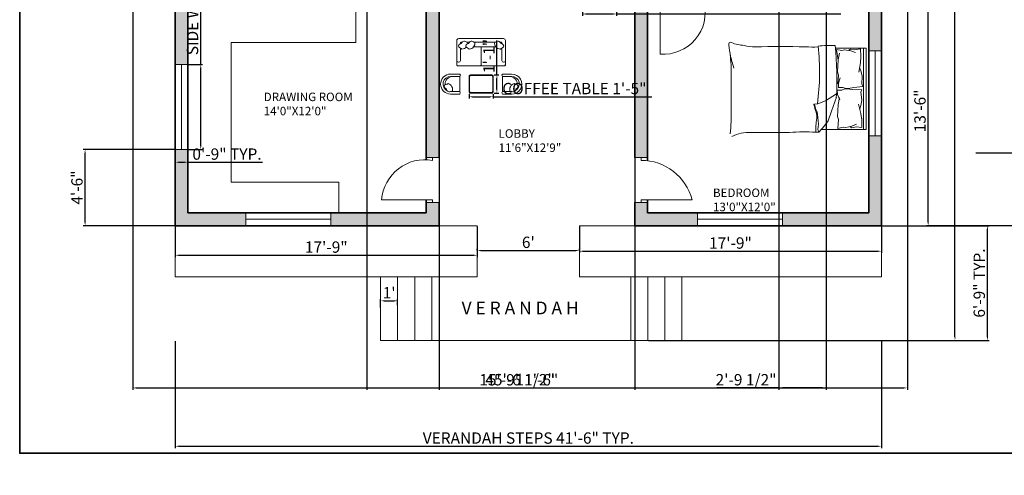
# Model space of a CAD drawing. Units: inches. Extents: x 2257 to 3678, y 834 to 1975.
# Tile 1 of 16: x 2257 to 2952, y 834 to 1155. Entities that reach past the tile are written whole.
import ezdxf

# ---------------------------------------------------------------- set-up
doc = ezdxf.new("R2010")
doc.units = ezdxf.units.IN
for name, color, linetype, lineweight in [('A-ANNO-DIMS', 2, 'Continuous', 18), ('A-ANNO-SYMB', 7, 'Continuous', 25), ('A-ANNO-TTLB', 7, 'Continuous', 35), ('A-AREA-IDEN', 7, 'Continuous', 18), ('A-DOOR', 3, 'Continuous', 18), ('A-FLOR-CASE', 8, 'Continuous', 18), ('A-FLOR-STRS', 7, 'Continuous', 18), ('A-FURN', 8, 'Continuous', 18), ('A-GLAZ', 4, 'Continuous', 18), ('A-WALL', 7, 'Continuous', 35)]:
    doc.layers.add(name, color=color, linetype=linetype, lineweight=lineweight)
doc.layers.add('A-WALL-PATT', color=251, linetype='Continuous', lineweight=13, true_color=0x636466)
doc.styles.get("Standard").update_dxf_attribs({"font": 'arial.ttf'})
doc.dimstyles.new('ISO-25', dxfattribs={"dimtxt": 8, "dimasz": 2.5, "dimexe": 1.25, "dimexo": 0.625, "dimtad": 1, "dimdec": 0, "dimlunit": 3, "dimtxsty": 'Standard', "dimcen": 2.5, "dimadec": 0, "dimazin": 0, "dimtfac": 1, "dimtdec": 0, "dimtmove": 0, "dimatfit": 3, "dimfxl": 1, "dimarcsym": 0})

# ---------------------------------------------------------------- blocks, each defined once
blk = doc.blocks.new('*D7')
at = {"layer": 'A-ANNO-DIMS', "color": 0, "lineweight": -2, "transparency": 16777216}
for p, q in [((2367.05, 1009.45), (2367.05, 987.96)), ((2580.05, 1009.45), (2580.05, 987.96)), ((2369.55, 989.21), (2577.55, 989.21))]:
    blk.add_line(p, q, dxfattribs=at)
at = {"layer": 'A-ANNO-DIMS', "color": 0, "transparency": 16777216}
for points in [[(2369.55, 989.62), (2369.55, 988.79), (2367.05, 989.21)], [(2577.55, 989.62), (2577.55, 988.79), (2580.05, 989.21)]]:
    blk.add_solid(points, dxfattribs=at)
at = {"layer": 'Defpoints', "color": 0, "transparency": 16777216}
for p in [(2367.05, 1010.08), (2580.05, 1010.08), (2580.05, 989.21)]:
    blk.add_point(p, dxfattribs=at)
at = {"layer": 'A-ANNO-DIMS', "color": 0, "transparency": 16777216, "insert": (2473.55, 993.92), "char_height": 8, "attachment_point": 5}
blk.add_mtext('17\'-9"', dxfattribs=at)
blk = doc.blocks.new('*D8')
at = {"layer": 'A-ANNO-DIMS', "color": 0, "lineweight": -2, "transparency": 16777216}
for p, q in [((2652.05, 1009.45), (2652.05, 990.83)), ((2865.05, 1009.45), (2865.05, 990.83)), ((2654.55, 992.08), (2862.55, 992.08))]:
    blk.add_line(p, q, dxfattribs=at)
at = {"layer": 'A-ANNO-DIMS', "color": 0, "transparency": 16777216}
for points in [[(2654.55, 992.49), (2654.55, 991.66), (2652.05, 992.08)], [(2862.55, 992.49), (2862.55, 991.66), (2865.05, 992.08)]]:
    blk.add_solid(points, dxfattribs=at)
at = {"layer": 'Defpoints', "color": 0, "transparency": 16777216}
for p in [(2652.05, 1010.08), (2865.05, 1010.08), (2865.05, 992.08)]:
    blk.add_point(p, dxfattribs=at)
at = {"layer": 'A-ANNO-DIMS', "color": 0, "transparency": 16777216, "insert": (2758.55, 996.79), "char_height": 8, "attachment_point": 5}
blk.add_mtext('17\'-9"', dxfattribs=at)
blk = doc.blocks.new('*D9')
at = {"layer": 'A-ANNO-DIMS', "color": 0, "lineweight": -2, "transparency": 16777216}
for p, q in [((2580.05, 992.7), (2580.05, 993.82)), ((2652.05, 992.7), (2652.05, 993.82)), ((2582.55, 992.57), (2649.55, 992.57))]:
    blk.add_line(p, q, dxfattribs=at)
at = {"layer": 'A-ANNO-DIMS', "color": 0, "transparency": 16777216}
for points in [[(2582.55, 992.99), (2582.55, 992.16), (2580.05, 992.57)], [(2649.55, 992.99), (2649.55, 992.16), (2652.05, 992.57)]]:
    blk.add_solid(points, dxfattribs=at)
at = {"layer": 'Defpoints', "color": 0, "transparency": 16777216}
for p in [(2580.05, 992.08), (2652.05, 992.57), (2652.05, 992.08)]:
    blk.add_point(p, dxfattribs=at)
at = {"layer": 'A-ANNO-DIMS', "color": 0, "transparency": 16777216, "insert": (2616.05, 997.28), "char_height": 8, "attachment_point": 5}
blk.add_mtext("6'", dxfattribs=at)
blk = doc.blocks.new('A$C1352')
at = {"color": 0}
for points in [[(0.003, 0.053), (0.003, 0.553, -0.414214), (0.053, 0.603), (0.753, 0.603, -0.414214), (0.803, 0.553), (0.803, 0.053, -0.414214), (0.753, 0.003), (0.053, 0.003, -0.414214)], [(0.023, 0.053), (0.023, 0.553, -0.414214), (0.053, 0.583), (0.753, 0.583, -0.414214), (0.783, 0.553), (0.783, 0.053, -0.414214), (0.753, 0.023), (0.053, 0.023, -0.414214)]]:
    blk.add_lwpolyline(points, format="xyb", close=True, dxfattribs=at)
blk = doc.blocks.new('*D21')
at = {"layer": 'A-ANNO-DIMS', "color": 0, "lineweight": -2, "transparency": 16777216}
for p, q in [((2511.89, 952.22), (2511.89, 958.28)), ((2523.89, 953.88), (2523.89, 958.28)), ((2514.39, 957.03), (2521.39, 957.03))]:
    blk.add_line(p, q, dxfattribs=at)
at = {"layer": 'A-ANNO-DIMS', "color": 0, "transparency": 16777216}
for points in [[(2514.39, 957.45), (2514.39, 956.61), (2511.89, 957.03)], [(2521.39, 957.45), (2521.39, 956.61), (2523.89, 957.03)]]:
    blk.add_solid(points, dxfattribs=at)
at = {"layer": 'Defpoints', "color": 0, "transparency": 16777216}
for p in [(2511.89, 951.59), (2523.89, 957.03), (2523.89, 953.26)]:
    blk.add_point(p, dxfattribs=at)
at = {"layer": 'A-ANNO-DIMS', "color": 0, "transparency": 16777216, "insert": (2517.89, 961.67), "char_height": 8, "attachment_point": 5}
blk.add_mtext("1'", dxfattribs=at)
blk = doc.blocks.new('BED-DOUBLE-PLAN')
for p, q in [((33.26, 63.38), (29.37, 58.94)), ((35.36, 63.48), (33.26, 63.38, 4.64)), ((34.01, 61.54), (33.26, 63.38)), ((0, 61.46), (31.9, 61.46)), ((0, 4.17), (0, 61.46)), ((1.84, 4.17), (1.84, 61.46)), ((3.07, 60.08), (2.95, 53.6)), ((3.07, 60.08), (6.92, 59.62)), ((9.9, 59.11), (6.69, 57.7)), ((6.92, 59.62), (10, 60.34)), ((14.18, 60.08), (9.9, 59.11)), ((10, 60.34), (11.25, 59.72)), ((16.11, 59.85), (14.18, 60.08)), ((19.87, 60.78), (16.11, 59.85)), ((19.38, 54.63), (19.87, 60.78)), ((29.37, 58.94), (26.77, 55.41)), ((33.63, 57.82), (34.01, 61.54)), ((34.01, 53.18), (33.63, 57.82)), ((2.95, 53.6), (3.05, 54.8)), ((3.05, 54.8), (3.68, 50.25)), ((3.68, 50.25), (5.3, 43.75)), ((20.05, 52.28), (19.38, 54.63)), ((19.54, 43.87), (20.05, 52.28)), ((24.36, 48.73), (20.84, 38.73)), ((26.77, 55.41), (24.36, 48.73)), ((34.56, 49.1), (34.01, 53.18)), ((35.68, 46.68), (34.56, 49.1)), ((3.69, 44.52), (3.04, 41.01)), ((4.4, 47), (3.69, 44.52)), ((18.74, 39.04), (19.54, 43.87)), ((28.62, 41.3), (34.01, 43.34)), ((34.01, 43.34), (36.42, 43.71)), ((36.42, 43.71), (35.68, 46.68)), ((95, 18.06), (95, 47.57)), ((3.57, 35.31), (2.99, 33.54)), ((3.04, 41.01), (3.07, 40.62)), ((3.07, 40.62), (3.57, 35.31)), ((20.07, 36.86), (18.53, 40.55)), ((20.25, 33.92), (20.07, 36.86)), ((20.84, 36.28), (28.62, 41.3)), ((2.24, 31.15), (8.66, 31.84)), ((2.94, 29.42), (2.24, 31.15)), ((2.76, 24.09), (2.94, 29.42)), ((2.99, 33.54), (9.43, 33.25)), ((8.66, 31.84), (12.47, 32.54)), ((9.43, 33.25), (13.28, 32.79)), ((12.47, 32.54), (14.03, 32.54)), ((13.28, 32.79), (14.84, 32.89)), ((14.03, 32.54), (16.28, 31.84)), ((14.84, 32.89), (17.04, 33.72)), ((16.28, 31.84), (19.5, 31.84)), ((17.04, 33.72), (20.25, 33.92)), ((19.5, 28.9), (18.19, 25.13)), ((19.38, 23.24), (19.87, 29.39)), ((19.5, 31.84), (19.5, 28.9)), ((2.76, 23.7), (2.76, 24.09)), ((3.63, 20.23), (2.76, 23.7)), ((3.98, 14.52), (5.19, 21.1)), ((20.05, 20.89), (19.38, 23.24)), ((19.54, 12.48), (20.05, 20.89)), ((4.5, 17.81), (3.63, 20.23)), ((3.63, 9.93), (3.98, 14.52)), ((3.61, 9.81), (3.63, 9.93)), ((4, 4.67), (3.61, 9.81)), ((10.74, 6.06), (7.44, 7.27)), ((18.74, 7.65), (19.54, 12.48)), ((19.54, 12.48), (19.92, 11.13)), ((19.92, 11.13), (20.79, 5.02)), ((21.71, 4.17), (0, 4.17)), ((3.98, 4.67), (7.79, 5.36)), ((7.79, 5.36), (10.91, 4.84)), ((15.07, 5.36), (10.74, 6.06)), ((10.91, 4.84), (12.12, 5.54)), ((16.98, 5.71), (15.07, 5.36)), ((20.79, 5.02), (16.98, 5.71))]:
    blk.add_line(p, q)
for centre, radius, start, end in [((-7.98, 61.53), 43.38, 349.87628, 2.56571), ((43.54, 218.51), 155.25, 266.97912, 273.83645), ((81.31, -5405.34), 5469.02, 90.00217, 90.28689), ((82.32, 91.3), 27.65, 267.47136, 296.46809), ((254.49, 49.33), 159.5, 174.4998, 180.63509), ((42.04, 52.44), 7.46, 168.6608, 203.73842), ((1.78, 37.35), 35.55, 10.66171, 19.88058), ((187.4, 21.29), 154.68, 171.78449, 186.90062), ((36.49, 43.92), 0.221, 250.24637, 1.13765), ((218.26, 25.61), 197.77, 176.08655, 186.78213), ((-28.43, -20.65), 127.63, 13.38322, 17.70533), ((240.78, 25.69), 145.97, 182.99578, 189.40907), ((24.09, 102.1), 99.87, 268.72178, 275.60397), ((37.37, -200.58), 203.94, 88.4762, 91.00819), ((60.68, 581.23), 578.22, 268.22771, 271.71854), ((77.34, -32.25), 35.53, 76.06484, 88.91125), ((84.25, -25.97), 28.25, 67.97508, 86.652), ((95.57, 1.3), 1.31, 236.17358, 23.47814)]:
    blk.add_arc(centre, radius, start, end)
blk = doc.blocks.new('WIN-60')
for p, q in [((0, 9), (0, 0)), ((60, 4.5), (60, 9)), ((60, 9), (60, 0)), ((0, 0), (0, 4.5)), ((0, 4.5), (60, 4.5))]:
    blk.add_line(p, q)
blk = doc.blocks.new('WIN-60-SIDE')
for p, q in [((0, 60), (9, 60)), ((9, 60), (4.5, 60)), ((4.5, 60), (4.5, 0)), ((9, 0), (0, 0)), ((4.5, 0), (9, 0))]:
    blk.add_line(p, q)
blk = doc.blocks.new('DOOR-BEDROOM-FRONT')
for p, q in [((0, 41.01), (0, 32.01)), ((0, 36.08), (2, 36.08)), ((2, 36.08), (2, 0.08)), ((34.84, 36.51), (32.84, 36.51)), ((34.84, 41.01), (34.84, 32.01)), ((34.84, 32.01), (34.84, 36.51))]:
    blk.add_line(p, q)
blk.add_arc((4.15, 29.52), 29.53, 265.82197, 13.68707)
blk = doc.blocks.new('DOOR-DRAWING-ROOM')
for p, q in [((31.5, 31.83), (40.5, 31.83)), ((40.5, 31.83), (36, 31.83)), ((36, 31.83), (36, 29.83)), ((36, 2), (0, 2)), ((36, 0), (36, 2)), ((31.5, 0), (40.5, 0)), ((40.5, 0), (36, 0))]:
    blk.add_line(p, q)
blk.add_arc((30.7, -0.52), 30.81, 80.10035, 175.31629)
blk = doc.blocks.new('DOOR-LOBBY-BEDROOM')
for p, q in [((0, 31.83), (9, 31.83)), ((9, 31.83), (4.5, 31.83)), ((4.5, 31.83), (4.5, 29.83)), ((4.5, 0), (4.5, 2)), ((4.5, 2), (40.5, 2)), ((0, 0), (0, 0)), ((0, 0), (9, 0)), ((9, 0), (4.5, 0))]:
    blk.add_line(p, q)
blk.add_arc((4.5, -7.37), 37.2, 14.58337, 90)
blk = doc.blocks.new('STEPS-VERANDAH')
for p, q in [((0, 80.97), (213, 80.97)), ((0, 44.97), (0, 80.97)), ((0, 80.97), (0, 80.97)), ((213, 80.97), (213, 44.97)), ((213, 80.97), (213, 44.97)), ((498, 80.97), (285, 80.97)), ((285, 80.97), (285, 44.97)), ((285, 80.97), (285, 44.97)), ((498, 44.97), (498, 80.97)), ((213, 44.97), (0, 44.97)), ((144.84, 0), (144.84, 44.97)), ((168.84, 44.97), (156.84, 44.97)), ((156.84, 44.97), (156.84, 0)), ((168.84, 0), (168.84, 44.97)), ((168.84, 44.97), (168.84, 44.97)), ((180.84, 44.97), (180.84, 0)), ((285, 44.97), (498, 44.97)), ((333.2, 44.97), (321.2, 44.97)), ((321.2, 44.97), (321.2, 0)), ((333.2, 0), (333.2, 44.97)), ((357.2, 44.97), (345.2, 44.97)), ((345.2, 44.97), (345.2, 0)), ((357.2, 0), (357.2, 44.97)), ((213, 0), (144.84, 0)), ((156.84, 0), (144.84, 0)), ((180.84, 0), (168.84, 0)), ((213, 0), (357.2, 0)), ((345.2, 0), (333.2, 0))]:
    blk.add_line(p, q)
blk = doc.blocks.new('*D54')
at = {"layer": 'A-ANNO-DIMS', "color": 0, "lineweight": -2, "transparency": 16777216}
for p, q in [((2574.2, 1102.98), (2574.2, 1099.79)), ((2576.7, 1101.04), (2588.83, 1101.04)), ((2591.33, 1102.98), (2591.33, 1099.79)), ((2591.33, 1101.04), (2703.2, 1101.04))]:
    blk.add_line(p, q, dxfattribs=at)
at = {"layer": 'A-ANNO-DIMS', "color": 0, "transparency": 16777216}
for points in [[(2576.7, 1101.45), (2576.7, 1100.62), (2574.2, 1101.04)], [(2588.83, 1101.45), (2588.83, 1100.62), (2591.33, 1101.04)]]:
    blk.add_solid(points, dxfattribs=at)
at = {"layer": 'Defpoints', "color": 0, "transparency": 16777216}
for p in [(2574.2, 1103.61), (2591.33, 1103.61), (2591.33, 1101.04)]:
    blk.add_point(p, dxfattribs=at)
at = {"layer": 'A-ANNO-DIMS', "color": 0, "transparency": 16777216, "insert": (2648.51, 1105.8), "char_height": 8, "attachment_point": 5}
blk.add_mtext('COFFEE TABLE 1\'-5"', dxfattribs=at)
blk = doc.blocks.new('*D55')
at = {"layer": 'A-ANNO-DIMS', "color": 0, "lineweight": -2, "transparency": 16777216}
for p, q in [((2593.9, 1116.46), (2593.9, 1140.72)), ((2591.96, 1116.46), (2595.15, 1116.46)), ((2593.9, 1106.11), (2593.9, 1113.96)), ((2591.96, 1103.61), (2595.15, 1103.61))]:
    blk.add_line(p, q, dxfattribs=at)
at = {"layer": 'A-ANNO-DIMS', "color": 0, "transparency": 16777216}
for points in [[(2593.49, 1113.96), (2594.32, 1113.96), (2593.9, 1116.46)], [(2593.49, 1106.11), (2594.32, 1106.11), (2593.9, 1103.61)]]:
    blk.add_solid(points, dxfattribs=at)
at = {"layer": 'Defpoints', "color": 0, "transparency": 16777216}
for p in [(2591.33, 1116.46), (2593.9, 1116.46), (2591.33, 1103.61)]:
    blk.add_point(p, dxfattribs=at)
at = {"layer": 'A-ANNO-DIMS', "color": 0, "transparency": 16777216, "insert": (2589.26, 1129.84), "char_height": 8, "attachment_point": 5, "rotation": 90}
blk.add_mtext('1\'-1"', dxfattribs=at)
blk = doc.blocks.new('*D58')
at = {"layer": 'A-ANNO-DIMS', "color": 0, "lineweight": -2, "transparency": 16777216}
for p, q in [((2385.05, 1123.86), (2385.05, 1257.67)), ((2376.68, 1123.86), (2386.3, 1123.86)), ((2385.05, 1066.36), (2385.05, 1121.36)), ((2376.68, 1063.86), (2386.3, 1063.86))]:
    blk.add_line(p, q, dxfattribs=at)
at = {"layer": 'A-ANNO-DIMS', "color": 0, "transparency": 16777216}
for points in [[(2384.63, 1121.36), (2385.47, 1121.36), (2385.05, 1123.86)], [(2384.63, 1066.36), (2385.47, 1066.36), (2385.05, 1063.86)]]:
    blk.add_solid(points, dxfattribs=at)
at = {"layer": 'Defpoints', "color": 0, "transparency": 16777216}
for p in [(2376.05, 1123.86), (2385.05, 1123.86), (2376.05, 1063.86)]:
    blk.add_point(p, dxfattribs=at)
at = {"layer": 'A-ANNO-DIMS', "color": 0, "transparency": 16777216, "insert": (2380.29, 1192.01), "char_height": 8, "attachment_point": 5, "rotation": 90}
blk.add_mtext('SIDE WINDOW 5\'-0" TYP.', dxfattribs=at)
blk = doc.blocks.new('*D59')
at = {"layer": 'A-ANNO-DIMS', "color": 0, "lineweight": -2, "transparency": 16777216}
for p, q in [((2367.05, 1063.23), (2367.05, 1053.61)), ((2376.05, 1063.23), (2376.05, 1053.61)), ((2369.55, 1054.86), (2373.55, 1054.86)), ((2376.05, 1054.86), (2428.56, 1054.86))]:
    blk.add_line(p, q, dxfattribs=at)
at = {"layer": 'A-ANNO-DIMS', "color": 0, "transparency": 16777216}
for points in [[(2369.55, 1055.28), (2369.55, 1054.44), (2367.05, 1054.86)], [(2373.55, 1055.28), (2373.55, 1054.44), (2376.05, 1054.86)]]:
    blk.add_solid(points, dxfattribs=at)
at = {"layer": 'Defpoints', "color": 0, "transparency": 16777216}
for p in [(2367.05, 1063.86), (2376.05, 1063.86), (2376.05, 1054.86)]:
    blk.add_point(p, dxfattribs=at)
at = {"layer": 'A-ANNO-DIMS', "color": 0, "transparency": 16777216, "insert": (2403.56, 1059.57), "char_height": 8, "attachment_point": 5}
blk.add_mtext('0\'-9" TYP.', dxfattribs=at)
blk = doc.blocks.new('*D60')
at = {"layer": 'A-ANNO-DIMS', "color": 0, "lineweight": -2, "transparency": 16777216}
for p, q in [((2654.22, 1162.45), (2654.22, 1158.23)), ((2656.72, 1159.48), (2675.72, 1159.48)), ((2678.22, 1162.45), (2678.22, 1158.23)), ((2678.22, 1159.48), (2836.5, 1159.48))]:
    blk.add_line(p, q, dxfattribs=at)
at = {"layer": 'A-ANNO-DIMS', "color": 0, "transparency": 16777216}
for points in [[(2656.72, 1159.89), (2656.72, 1159.06), (2654.22, 1159.48)], [(2675.72, 1159.89), (2675.72, 1159.06), (2678.22, 1159.48)]]:
    blk.add_solid(points, dxfattribs=at)
at = {"layer": 'Defpoints', "color": 0, "transparency": 16777216}
for p in [(2654.22, 1163.08), (2678.22, 1163.08), (2678.22, 1159.48)]:
    blk.add_point(p, dxfattribs=at)
at = {"layer": 'A-ANNO-DIMS', "color": 0, "transparency": 16777216, "insert": (2758.61, 1164.24), "char_height": 8, "attachment_point": 5}
blk.add_mtext('NARROW WINDOW 2\'-0" TYP.', dxfattribs=at)
blk = doc.blocks.new('*D82')
at = {"layer": 'A-ANNO-DIMS', "color": 0, "lineweight": -2, "transparency": 16777216}
for p, q in [((2367.05, 928.48), (2367.05, 853.15)), ((2865.05, 928.48), (2865.05, 853.15)), ((2369.55, 854.4), (2862.55, 854.4))]:
    blk.add_line(p, q, dxfattribs=at)
at = {"layer": 'A-ANNO-DIMS', "color": 0, "transparency": 16777216}
for points in [[(2369.55, 854.82), (2369.55, 853.99), (2367.05, 854.4)], [(2862.55, 854.82), (2862.55, 853.99), (2865.05, 854.4)]]:
    blk.add_solid(points, dxfattribs=at)
at = {"layer": 'Defpoints', "color": 0, "transparency": 16777216}
for p in [(2367.05, 929.1), (2865.05, 929.1), (2865.05, 854.4)]:
    blk.add_point(p, dxfattribs=at)
at = {"layer": 'A-ANNO-DIMS', "color": 0, "transparency": 16777216, "insert": (2616.05, 859.16), "char_height": 8, "attachment_point": 5}
blk.add_mtext('VERANDAH STEPS 41\'-6" TYP.', dxfattribs=at)
blk = doc.blocks.new('*D83')
at = {"layer": 'A-ANNO-DIMS', "color": 0, "lineweight": -2, "transparency": 16777216}
for p, q in [((2865.68, 1010.08), (2941, 1010.08)), ((2939.75, 931.6), (2939.75, 1007.58)), ((2865.68, 929.1), (2941, 929.1))]:
    blk.add_line(p, q, dxfattribs=at)
at = {"layer": 'A-ANNO-DIMS', "color": 0, "transparency": 16777216}
for points in [[(2939.33, 1007.58), (2940.17, 1007.58), (2939.75, 1010.08)], [(2939.33, 931.6), (2940.17, 931.6), (2939.75, 929.1)]]:
    blk.add_solid(points, dxfattribs=at)
at = {"layer": 'Defpoints', "color": 0, "transparency": 16777216}
for p in [(2865.05, 1010.08), (2939.75, 1010.08), (2865.05, 929.1)]:
    blk.add_point(p, dxfattribs=at)
at = {"layer": 'A-ANNO-DIMS', "color": 0, "transparency": 16777216, "insert": (2935.04, 969.59), "char_height": 8, "attachment_point": 5, "rotation": 90}
blk.add_mtext('6\'-9" TYP.', dxfattribs=at)
blk = doc.blocks.new('*D96')
at = {"layer": 'A-ANNO-DIMS', "color": 0, "lineweight": -2, "transparency": 16777216}
for p, q in [((2337.05, 1283.95), (2337.05, 894.3)), ((2883.34, 1168.45), (2883.34, 894.3)), ((2339.55, 895.55), (2880.84, 895.55))]:
    blk.add_line(p, q, dxfattribs=at)
at = {"layer": 'A-ANNO-DIMS', "color": 0, "transparency": 16777216}
for points in [[(2339.55, 895.97), (2339.55, 895.14), (2337.05, 895.55)], [(2880.84, 895.97), (2880.84, 895.14), (2883.34, 895.55)]]:
    blk.add_solid(points, dxfattribs=at)
at = {"layer": 'Defpoints', "color": 0, "transparency": 16777216}
for p in [(2337.05, 1284.58), (2883.34, 1169.08), (2883.34, 895.55)]:
    blk.add_point(p, dxfattribs=at)
at = {"layer": 'A-ANNO-DIMS', "color": 0, "transparency": 16777216, "insert": (2610.2, 900.31), "char_height": 8, "attachment_point": 5}
blk.add_mtext('45\'-6 1/2"', dxfattribs=at)
blk = doc.blocks.new('*D97')
at = {"layer": 'A-ANNO-DIMS', "color": 0, "lineweight": -2, "transparency": 16777216}
for p, q in [((2835.68, 1593.58), (2918.14, 1593.58)), ((2916.89, 931.6), (2916.89, 1591.08)), ((2700.87, 929.1), (2918.14, 929.1))]:
    blk.add_line(p, q, dxfattribs=at)
at = {"layer": 'A-ANNO-DIMS', "color": 0, "transparency": 16777216}
for points in [[(2916.47, 1591.08), (2917.31, 1591.08), (2916.89, 1593.58)], [(2916.47, 931.6), (2917.31, 931.6), (2916.89, 929.1)]]:
    blk.add_solid(points, dxfattribs=at)
at = {"layer": 'Defpoints', "color": 0, "transparency": 16777216}
for p in [(2835.05, 1593.58), (2916.89, 1593.58), (2700.25, 929.1)]:
    blk.add_point(p, dxfattribs=at)
at = {"layer": 'A-ANNO-DIMS', "color": 0, "transparency": 16777216, "insert": (2912.13, 1261.34), "char_height": 8, "attachment_point": 5, "rotation": 90}
blk.add_mtext('55\'-4 1/2"', dxfattribs=at)
blk = doc.blocks.new('*D101')
at = {"layer": 'A-ANNO-DIMS', "color": 0, "lineweight": -2, "transparency": 16777216}
for p, q in [((3136.62, 1172.08), (2896.72, 1172.08)), ((2897.97, 1012.58), (2897.97, 1169.58)), ((3010.62, 1010.08), (2896.72, 1010.08))]:
    blk.add_line(p, q, dxfattribs=at)
at = {"layer": 'A-ANNO-DIMS', "color": 0, "transparency": 16777216}
for points in [[(2897.55, 1169.58), (2898.38, 1169.58), (2897.97, 1172.08)], [(2897.55, 1012.58), (2898.38, 1012.58), (2897.97, 1010.08)]]:
    blk.add_solid(points, dxfattribs=at)
at = {"layer": 'Defpoints', "color": 0, "transparency": 16777216}
for p in [(2897.97, 1172.08), (3137.24, 1172.08), (3011.24, 1010.08)]:
    blk.add_point(p, dxfattribs=at)
at = {"layer": 'A-ANNO-DIMS', "color": 0, "transparency": 16777216, "insert": (2893.25, 1091.08), "char_height": 8, "attachment_point": 5, "rotation": 90}
blk.add_mtext('13\'-6"', dxfattribs=at)
blk = doc.blocks.new('*D106')
at = {"layer": 'A-ANNO-DIMS', "color": 0, "lineweight": -2, "transparency": 16777216}
for p, q in [((2553.05, 1583.95), (2553.05, 894.3)), ((2691.05, 1583.95), (2691.05, 894.3)), ((2555.55, 895.55), (2688.55, 895.55))]:
    blk.add_line(p, q, dxfattribs=at)
at = {"layer": 'A-ANNO-DIMS', "color": 0, "transparency": 16777216}
for points in [[(2555.55, 895.97), (2555.55, 895.14), (2553.05, 895.55)], [(2688.55, 895.97), (2688.55, 895.14), (2691.05, 895.55)]]:
    blk.add_solid(points, dxfattribs=at)
at = {"layer": 'Defpoints', "color": 0, "transparency": 16777216}
for p in [(2553.05, 1584.58), (2691.05, 1584.58), (2691.05, 895.55)]:
    blk.add_point(p, dxfattribs=at)
at = {"layer": 'A-ANNO-DIMS', "color": 0, "transparency": 16777216, "insert": (2622.05, 900.26), "char_height": 8, "attachment_point": 5}
blk.add_mtext('11\'-6"', dxfattribs=at)
blk = doc.blocks.new('*D107')
at = {"layer": 'A-ANNO-DIMS', "color": 0, "lineweight": -2, "transparency": 16777216}
for p, q in [((2502.05, 1430.95), (2502.05, 894.3)), ((2691.05, 1430.95), (2691.05, 894.3)), ((2504.55, 895.55), (2688.55, 895.55))]:
    blk.add_line(p, q, dxfattribs=at)
at = {"layer": 'A-ANNO-DIMS', "color": 0, "transparency": 16777216}
for points in [[(2504.55, 895.97), (2504.55, 895.14), (2502.05, 895.55)], [(2688.55, 895.97), (2688.55, 895.14), (2691.05, 895.55)]]:
    blk.add_solid(points, dxfattribs=at)
at = {"layer": 'Defpoints', "color": 0, "transparency": 16777216}
for p in [(2502.05, 1431.58), (2691.05, 1431.58), (2691.05, 895.55)]:
    blk.add_point(p, dxfattribs=at)
at = {"layer": 'A-ANNO-DIMS', "color": 0, "transparency": 16777216, "insert": (2596.55, 900.26), "char_height": 8, "attachment_point": 5}
blk.add_mtext('15\'-9"', dxfattribs=at)
blk = doc.blocks.new('*D112')
at = {"layer": 'A-ANNO-DIMS', "color": 0, "lineweight": -2, "transparency": 16777216}
for p, q in [((2366.43, 1063.86), (2302.25, 1063.86)), ((2303.5, 1012.58), (2303.5, 1061.36)), ((2366.43, 1010.08), (2302.25, 1010.08))]:
    blk.add_line(p, q, dxfattribs=at)
at = {"layer": 'A-ANNO-DIMS', "color": 0, "transparency": 16777216}
for points in [[(2303.08, 1061.36), (2303.92, 1061.36), (2303.5, 1063.86)], [(2303.08, 1012.58), (2303.92, 1012.58), (2303.5, 1010.08)]]:
    blk.add_solid(points, dxfattribs=at)
at = {"layer": 'Defpoints', "color": 0, "transparency": 16777216}
for p in [(2303.5, 1063.86), (2367.05, 1063.86), (2367.05, 1010.08)]:
    blk.add_point(p, dxfattribs=at)
at = {"layer": 'A-ANNO-DIMS', "color": 0, "transparency": 16777216, "insert": (2298.79, 1036.97), "char_height": 8, "attachment_point": 5, "rotation": 90}
blk.add_mtext('4\'-6"', dxfattribs=at)
blk = doc.blocks.new('*D117')
at = {"layer": 'A-ANNO-DIMS', "color": 0, "lineweight": -2, "transparency": 16777216}
for p, q in [((2792.7, 1439.95), (2792.7, 894.3)), ((2826.05, 1439.95), (2826.05, 894.3)), ((2792.7, 895.55), (2748.91, 895.55)), ((2823.55, 895.55), (2795.2, 895.55))]:
    blk.add_line(p, q, dxfattribs=at)
at = {"layer": 'A-ANNO-DIMS', "color": 0, "transparency": 16777216}
for points in [[(2795.2, 895.97), (2795.2, 895.14), (2792.7, 895.55)], [(2823.55, 895.97), (2823.55, 895.14), (2826.05, 895.55)]]:
    blk.add_solid(points, dxfattribs=at)
at = {"layer": 'Defpoints', "color": 0, "transparency": 16777216}
for p in [(2792.7, 1440.58), (2826.05, 1440.58), (2792.7, 895.55)]:
    blk.add_point(p, dxfattribs=at)
at = {"layer": 'A-ANNO-DIMS', "color": 0, "transparency": 16777216, "insert": (2769.55, 900.31), "char_height": 8, "attachment_point": 5}
blk.add_mtext('2\'-9 1/2"', dxfattribs=at)

msp = doc.modelspace()

# ---------------------------------------------------------------- hatches: boundary and pattern name
at = {"layer": 'A-WALL-PATT'}
h = msp.add_hatch(color=256, dxfattribs=at)
h.dxf.hatch_style = 1
h.paths.add_polyline_path([(2736.02, 1589.08), (2736.02, 1593.58), (2691.05, 1593.58), (2648.2, 1593.58), (2648.2, 1584.58), (2691.05, 1584.58), (2691.05, 1485.58), (2700.05, 1485.58), (2700.05, 1584.58), (2736.02, 1584.58)])
h.paths.add_polyline_path([(2835.05, 1593.58), (2796.02, 1593.58), (2796.02, 1584.58), (2826.05, 1584.58), (2826.05, 1440.58), (2835.05, 1440.58)])
h.paths.add_polyline_path([(2865.05, 1440.58), (2826.05, 1440.58), (2700.05, 1440.58), (2691.05, 1440.58), (2691.05, 1431.58), (2691.05, 1284.58), (2700.05, 1284.58), (2700.05, 1431.58), (2826.05, 1431.58), (2856.05, 1431.58), (2856.05, 1395.2), (2865.05, 1395.2), (2865.05, 1431.58)])
h.paths.add_polyline_path([(2865.05, 1335.2), (2856.05, 1335.2), (2856.05, 1293.58), (2741.94, 1293.58), (2741.94, 1289.08), (2741.94, 1284.58), (2865.05, 1284.58)], flags=17)
h.paths.add_polyline_path([(2865.05, 1172.08), (2856.05, 1172.08), (2741.94, 1172.08), (2741.94, 1163.08), (2856.05, 1163.08), (2856.05, 1133.53), (2865.05, 1133.53)])
h.paths.add_polyline_path([(2865.05, 1073.53), (2856.05, 1073.53), (2856.05, 1019.08), (2795.28, 1019.08), (2795.28, 1010.08), (2865.05, 1010.08)])
h.paths.add_polyline_path([(2735.28, 1014.58), (2735.28, 1019.08), (2700.05, 1019.08), (2700.05, 1026.35), (2695.55, 1026.35), (2691.05, 1026.35), (2691.05, 1010.08), (2735.28, 1010.08)])
h.paths.add_polyline_path([(2700.05, 1163.08), (2700.05, 1172.08), (2691.05, 1172.08), (2685.7, 1172.08), (2685.7, 1163.08), (2691.05, 1163.08), (2691.05, 1058.19), (2700.05, 1058.19)])
h.paths.add_polyline_path([(2707.1, 1172.08), (2700.05, 1172.08), (2700.05, 1163.08), (2707.1, 1163.08)])
h.paths.add_polyline_path([(2685.7, 1172.08), (2678.22, 1172.08), (2678.22, 1163.08), (2685.7, 1163.08)])
h.paths.add_polyline_path([(2654.22, 1172.08), (2648.96, 1172.08), (2648.96, 1163.08), (2654.22, 1163.08), (2654.22, 1167.58)])
h.paths.add_polyline_path([(2553.05, 1163.08), (2558.66, 1163.08), (2558.66, 1172.08), (2544.05, 1172.08), (2544.05, 1163.08), (2544.05, 1058.19), (2553.05, 1058.19)])
h.paths.add_polyline_path([(2568.8, 1167.58), (2568.8, 1172.08), (2558.66, 1172.08), (2558.66, 1163.08), (2568.8, 1163.08)])
h.paths.add_polyline_path([(2596.82, 1172.08), (2592.8, 1172.08), (2592.8, 1163.08), (2596.82, 1163.08)])
h.paths.add_polyline_path([(2553.05, 1019.08), (2553.05, 1026.35), (2548.55, 1026.35), (2544.05, 1026.35), (2544.05, 1019.08), (2476.8, 1019.08), (2476.8, 1010.08), (2553.05, 1010.08)])
h.paths.add_polyline_path([(2376.05, 1163.08), (2502.05, 1163.08), (2502.05, 1172.08), (2446.55, 1172.08), (2446.55, 1195.52), (2446.55, 1215.32), (2442.05, 1215.32), (2442.05, 1195.52), (2442.05, 1172.08), (2412.05, 1172.08), (2412.05, 1167.58), (2376.05, 1167.58), (2376.05, 1172.08), (2376.05, 1201.28), (2367.05, 1201.28), (2367.05, 1172.08), (2367.05, 1123.86), (2376.05, 1123.86)])
h.paths.add_polyline_path([(2577.05, 1440.58), (2376.05, 1440.58), (2376.05, 1485.89), (2367.05, 1485.89), (2367.05, 1440.58), (2337.05, 1440.58), (2337.05, 1403.59), (2346.05, 1403.59), (2346.05, 1431.58), (2493.05, 1431.58), (2493.05, 1293.58), (2484.41, 1293.58), (2484.41, 1284.58), (2502.05, 1284.58), (2502.05, 1431.58), (2577.05, 1431.58)])
h.paths.add_polyline_path([(2346.05, 1343.59), (2337.05, 1343.59), (2337.05, 1284.58), (2448.12, 1284.58), (2448.12, 1289.08), (2448.12, 1293.58), (2346.05, 1293.58)], flags=17)
h.paths.add_polyline_path([(2376.05, 1244.08), (2446.55, 1244.08), (2446.55, 1248.58), (2367.05, 1248.58), (2367.05, 1225.28), (2375.64, 1225.28), (2375.64, 1228.02), (2376.05, 1228.02)])
h.paths.add_polyline_path([(2588.2, 1589.08), (2588.2, 1593.58), (2468.1, 1593.58), (2468.1, 1584.58), (2544.05, 1584.58), (2544.05, 1541.08), (2568.05, 1541.08), (2568.05, 1490.08), (2544.05, 1490.08), (2544.05, 1485.58), (2577.05, 1485.58), (2577.05, 1545.58), (2553.05, 1545.58), (2553.05, 1584.58), (2588.2, 1584.58)])
h.paths.add_polyline_path([(2376.05, 1584.58), (2408.1, 1584.58), (2408.1, 1589.08), (2408.1, 1593.58), (2367.05, 1593.58), (2367.05, 1545.89), (2376.05, 1545.89)])
h.paths.add_polyline_path([(2376.05, 1063.86), (2367.05, 1063.86), (2367.05, 1019.08), (2367.05, 1010.08), (2416.8, 1010.08), (2416.8, 1014.58), (2416.8, 1019.08), (2376.05, 1019.08)])

# ---------------------------------------------------------------- linework, layer by layer
at = {"layer": 'A-ANNO-SYMB'}
msp.add_line((2931.52, 1061.57), (3577.66, 1061.57), dxfattribs=at)
at = {"layer": 'A-ANNO-TTLB'}
msp.add_lwpolyline([(2257.38, 1974.9), (3677.96, 1974.9), (3677.96, 849.42), (2257.38, 849.42)], close=True, dxfattribs=at)
at = {"layer": 'A-FLOR-CASE'}
for p, q in [((2494.46, 1139.28), (2494.46, 1163.08)), ((2478.15, 1139.28), (2406.54, 1139.28)), ((2406.54, 1139.28), (2406.54, 1040.73)), ((2478.15, 1139.28), (2494.46, 1139.28)), ((2406.54, 1040.73), (2482.31, 1040.73)), ((2482.31, 1040.73), (2482.31, 1019.08))]:
    msp.add_line(p, q, dxfattribs=at)
at = {"layer": 'A-FURN'}
for p, q in [((2568.2, 1138.56), (2568.2, 1139.16)), ((2568.63, 1139.59), (2569.42, 1139.59)), ((2574.56, 1139.59), (2572.51, 1139.59)), ((2573.77, 1139.59), (2574.56, 1139.59)), ((2593.02, 1139.59), (2577.65, 1139.59)), ((2596.9, 1139.59), (2596.11, 1139.59)), ((2597.33, 1138.56), (2597.33, 1139.16)), ((2568.2, 1135.31), (2568.2, 1126.74)), ((2597.33, 1126.74), (2597.33, 1135.31)), ((2561.23, 1104.68), (2567.77, 1104.68)), ((2604.3, 1104.68), (2597.76, 1104.68))]:
    msp.add_line(p, q, dxfattribs=at)
at = {"layer": 'A-FURN', "ltscale": 0.03}
msp.add_lwpolyline([(2582.78, 1123.74, 0.414214), (2583.63, 1122.88), (2599.04, 1122.88, 0.414214), (2599.9, 1123.74), (2599.9, 1140.87, 0.414214), (2598.61, 1142.16), (2566.92, 1142.16, 0.414214), (2565.63, 1140.87), (2565.63, 1123.74, 0.414214), (2566.49, 1122.88), (2581.9, 1122.88, 0.414214), (2582.75, 1123.74)], format="xyb", dxfattribs=at)
at = {"layer": 'A-FURN'}
for points in [[(2577.48, 1136.27), (2581.69, 1136.27, -0.414214), (2582.77, 1135.2), (2582.77, 1123.95, -0.414214), (2581.69, 1122.88), (2566.7, 1122.88, -0.414214), (2565.63, 1123.95)], [(2592.46, 1136.27), (2583.84, 1136.27, 0.414214), (2582.77, 1135.2), (2582.77, 1123.95, 0.414214), (2583.84, 1122.88), (2598.83, 1122.88, 0.414214), (2599.9, 1123.95)], [(2558.77, 1105.29, -0.785087), (2561.24, 1115.39), (2567.78, 1115.39)], [(2606.76, 1105.29, 0.785087), (2604.29, 1115.39), (2597.75, 1115.39)]]:
    msp.add_lwpolyline(points, format="xyb", dxfattribs=at)
msp.add_lwpolyline([(2577.48, 1136.27), (2593.19, 1136.27)], dxfattribs=at)
at = {"layer": 'A-FURN', "ltscale": 0.03}
for points in [[(2567.77, 1104.68, -0.369229), (2567.77, 1102.97), (2561.23, 1102.97, -1), (2561.25, 1117.11), (2567.78, 1117.1, -0.369229), (2567.78, 1115.39)], [(2597.76, 1104.68, 0.369229), (2597.76, 1102.97), (2604.3, 1102.97, 1), (2604.28, 1117.11), (2597.75, 1117.1, 0.369229), (2597.75, 1115.39)]]:
    msp.add_lwpolyline(points, format="xyb", close=True, dxfattribs=at)
at = {"layer": 'A-FURN'}
for centre, radius, start, end in [((2569.1, 1136.32), 2.42, 94.54394, 160.89739), ((2568.63, 1139.16), 0.428, 90, 180), ((2568.63, 1139.16), 0.428, 90, 180), ((2570.96, 1138.1), 2.15, 41.75724, 162.9051), ((2574.25, 1136.32), 2.42, 94.54394, 160.89739), ((2569.13, 1138.9), 4.15, 354.88098, 8.88305), ((2576.11, 1138.1), 2.15, 41.75724, 162.9051), ((2574.28, 1138.9), 4.15, 271.61163, 8.88305), ((2596.4, 1138.9), 4.15, 171.11695, 268.38837), ((2594.57, 1138.1), 2.15, 17.0949, 138.24276), ((2596.43, 1136.32), 2.42, 19.10261, 85.45606), ((2596.9, 1139.16), 0.428, 0, 90), ((2569.01, 1137.36), 2.2, 186.42786, 269.257), ((2569.18, 1135), 0.256, 142.15499, 285.27353), ((2569.13, 1138.9), 4.15, 271.61163, 319.37599), ((2574.15, 1137.36), 2.2, 186.42786, 269.257), ((2574.32, 1135), 0.256, 142.15499, 285.27353), ((2596.35, 1135), 0.256, 254.72647, 37.84501), ((2596.52, 1137.36), 2.2, 270.743, 353.57214), ((2566.92, 1126.74), 1.28, 180, 270), ((2566.92, 1126.74), 1.28, 270, 0), ((2598.61, 1126.74), 1.28, 180, 270), ((2598.61, 1126.74), 1.28, 270, 0), ((2562.75, 1110.04), 5.35, 89.94615, 183.65802), ((2602.78, 1110.04), 5.35, 356.34198, 90.05385), ((2558.67, 1107.89), 2.2, 76.64032, 159.46946), ((2559.02, 1108.87), 2.42, 184.99993, 251.35338), ((2560.39, 1106.7), 2.15, 182.99222, 304.14008), ((2559.41, 1110.14), 0.256, 60.62379, 203.74232), ((2558.42, 1106.37), 4.15, 337.01427, 74.28569), ((2561.24, 1110.04), 5.35, 268.85363, 269.94615), ((2607.11, 1106.37), 4.15, 105.71431, 202.98573), ((2605.14, 1106.7), 2.15, 235.85992, 357.00778), ((2604.29, 1110.04), 5.35, 270.05385, 271.14637), ((2606.12, 1110.14), 0.256, 336.25768, 119.37621), ((2606.86, 1107.89), 2.2, 20.53054, 103.35968), ((2606.51, 1108.87), 2.42, 288.64662, 355.00007)]:
    msp.add_arc(centre, radius, start, end, dxfattribs=at)
at = {"layer": 'A-GLAZ'}
msp.add_line((2416.8, 1014.58), (2416.8, 1014.58), dxfattribs=at)
at = {"layer": 'A-WALL'}
for p, q in [((2367.05, 1172.08), (2367.05, 1010.08)), ((2544.05, 1172.08), (2544.05, 1056.64)), ((2865.05, 1172.08), (2865.05, 1010.08)), ((2367.05, 1163.08), (2367.05, 1019.08)), ((2376.05, 1163.08), (2376.05, 1019.08)), ((2553.05, 1163.08), (2553.05, 1058.19)), ((2691.05, 1163.08), (2691.05, 1058.19)), ((2700.05, 1163.08), (2700.05, 1055.91)), ((2856.05, 1163.08), (2856.05, 1019.08)), ((2856.05, 1163.08), (2856.05, 1019.08)), ((2544.05, 1028.35), (2544.05, 1019.08)), ((2700.05, 1028.35), (2700.05, 1019.08)), ((2553.05, 1026.35), (2553.05, 1010.08)), ((2691.05, 1026.35), (2691.05, 1010.08)), ((2376.05, 1019.08), (2544.05, 1019.08)), ((2553.05, 1019.08), (2553.05, 1010.08)), ((2856.05, 1019.08), (2700.05, 1019.08)), ((2553.05, 1010.08), (2367.05, 1010.08)), ((2691.05, 1010.08), (2700.05, 1010.08)), ((2700.05, 1010.08), (2865.05, 1010.08))]:
    msp.add_line(p, q, dxfattribs=at)

# ---------------------------------------------------------------- block references
at = {"layer": 'A-DOOR'}
for name, p in [('DOOR-BEDROOM-FRONT', (2707.1, 1131.07)), ('DOOR-DRAWING-ROOM', (2512.55, 1026.36)), ('DOOR-LOBBY-BEDROOM', (2691.05, 1026.36))]:
    msp.add_blockref(name, p, dxfattribs=at)
at = {"layer": 'A-FLOR-STRS'}
msp.add_blockref('STEPS-VERANDAH', (2367.05, 929.1), dxfattribs=at)
at = {"layer": 'A-FURN', "rotation": 180}
msp.add_blockref('BED-DOUBLE-PLAN', (2854.16, 1139.53), dxfattribs=at)
at = {"layer": 'A-FURN', "ltscale": 0.03, "xscale": 21.41664423163014, "yscale": 21.41664423163014, "zscale": 21.41664423163014}
msp.add_blockref('A$C1352', (2574.14, 1103.54), dxfattribs=at)
at = {"layer": 'A-GLAZ', "extrusion": (0, 0, -1), "zscale": -1, "rotation": 269.9999999999992}
msp.add_blockref('WIN-60', (-2865.05, 1133.53), dxfattribs=at)
at = {"layer": 'A-GLAZ'}
for name, p in [('WIN-60-SIDE', (2367.05, 1063.86)), ('WIN-60', (2416.8, 1010.08)), ('WIN-60', (2735.28, 1010.08))]:
    msp.add_blockref(name, p, dxfattribs=at)

# ---------------------------------------------------------------- texts
at = {"layer": 'A-AREA-IDEN', "attachment_point": 1}
for s, width, insert, char_height in [('DRAWING ROOM\\P14\'0"X12\'0"', 270.6088, (2429.44, 1103.98), 6), ('LOBBY\\P11\'6"X12\'9"', 120.6846, (2595.02, 1078.11), 6), ('BEDROOM\\P13\'0"X12\'0"', 163.9638, (2746.23, 1036.3), 6), ('V E R A N D A H', 193.7314, (2568.98, 956.51), 9)]:
    msp.add_mtext_dynamic_manual_height_columns(s, width=width, gutter_width=12.5, heights=[0], dxfattribs=dict(at, insert=insert, char_height=char_height))

# ---------------------------------------------------------------- dimensions: what is measured, and where the dimension line sits
at = {"layer": 'A-ANNO-DIMS'}
for base, p1, p2, picture, middle in [((2916.89, 1593.58), (2700.25, 929.1), (2835.05, 1593.58), '*D97', (2912.13, 1261.34)), ((2897.97, 1172.08), (3011.24, 1010.08), (3137.24, 1172.08), '*D101', (2893.25, 1091.08)), ((2593.9018, 1116.45778), (2591.3318, 1103.60779), (2591.3318, 1116.45778), '*D55', (2589.26043, 1129.83926)), ((2303.5, 1063.86), (2367.05, 1010.08), (2367.05, 1063.86), '*D112', (2298.79, 1036.97))]:
    dim = msp.add_linear_dim(base=base, p1=p1, p2=p2, angle=90, dimstyle='ISO-25', override={"dimdec": 1, "dimlfac": 1, "dimrnd": 0, "dimzin": 1, "dimdsep": 46, "dimlunit": 4, "dimfrac": 2}, dxfattribs=at)
    dim.commit()
    dim.dimension.update_dxf_attribs({"geometry": picture, "text_midpoint": middle})
for base, p1, p2, override, picture, middle in [((2691.05, 895.55), (2553.05, 1584.58), (2691.05, 1584.58), {"dimdec": 1, "dimlfac": 1, "dimrnd": 0, "dimzin": 1, "dimdsep": 46, "dimlunit": 4, "dimfrac": 2}, '*D106', (2622.05, 900.26)), ((2792.699, 895.5533), (2826.0509, 1440.5769), (2792.699, 1440.5769), {"dimdec": 1, "dimlfac": 1, "dimrnd": 0, "dimzin": 1, "dimdsep": 46, "dimlunit": 4, "dimfrac": 2}, '*D117', (2769.5522, 900.3148)), ((2691.05, 895.55), (2502.05, 1431.58), (2691.05, 1431.58), {"dimdec": 1, "dimlfac": 1, "dimrnd": 0, "dimzin": 1, "dimdsep": 46, "dimlunit": 4, "dimfrac": 2}, '*D107', (2596.55, 900.26)), ((2883.34, 895.55), (2337.05, 1284.58), (2883.34, 1169.08), {"dimdec": 1, "dimlfac": 1, "dimrnd": 0, "dimzin": 1, "dimdsep": 46, "dimlunit": 4, "dimfrac": 2}, '*D96', (2610.2, 900.31)), ((2580.05, 989.21), (2367.05, 1010.08), (2580.05, 1010.08), {"dimclrd": 0, "dimclre": 0, "dimclrt": 0}, '*D7', (2473.55, 993.92)), ((2865.05, 992.08), (2652.05, 1010.08), (2865.05, 1010.08), {"dimclrd": 0, "dimclre": 0, "dimclrt": 0}, '*D8', (2758.55, 996.79)), ((2652.05, 992.57), (2580.05, 992.08), (2652.05, 992.08), {"dimclrd": 0, "dimclre": 0, "dimclrt": 0}, '*D9', (2616.05, 997.28)), ((2523.89, 957.03), (2511.89, 951.59), (2523.89, 953.26), {"dimclrd": 0, "dimclre": 0, "dimclrt": 0}, '*D21', (2517.89, 961.67))]:
    dim = msp.add_linear_dim(base=base, p1=p1, p2=p2, dimstyle='ISO-25', override=override, dxfattribs=at)
    dim.commit()
    dim.dimension.update_dxf_attribs({"geometry": picture, "text_midpoint": middle})
for base, p1, p2, text, picture, middle in [((2385.05, 1123.86), (2376.05, 1063.86), (2376.05, 1123.86), 'SIDE WINDOW <> TYP.', '*D58', (2380.29, 1192.01)), ((2939.75, 1010.08), (2865.05, 929.1), (2865.05, 1010.08), '<> TYP.', '*D83', (2935.04, 969.59))]:
    dim = msp.add_linear_dim(base=base, p1=p1, p2=p2, angle=90, text=text, dimstyle='ISO-25', override={"dimdec": 1, "dimlfac": 1, "dimrnd": 0, "dimzin": 1, "dimdsep": 46, "dimlunit": 4, "dimfrac": 2}, dxfattribs=at)
    dim.commit()
    dim.dimension.update_dxf_attribs({"geometry": picture, "text_midpoint": middle})
for base, p1, p2, text, picture, middle in [((2678.22, 1159.48), (2654.22, 1163.08), (2678.22, 1163.08), 'NARROW WINDOW <> TYP.', '*D60', (2758.61, 1164.24)), ((2591.33, 1101.04), (2574.2, 1103.61), (2591.33, 1103.61), 'COFFEE TABLE <>', '*D54', (2648.51, 1105.8)), ((2376.05, 1054.86), (2367.05, 1063.86), (2376.05, 1063.86), '<> TYP.', '*D59', (2403.56, 1059.57)), ((2865.05, 854.4), (2367.05, 929.1), (2865.05, 929.1), 'VERANDAH STEPS <> TYP.', '*D82', (2616.05, 859.16))]:
    dim = msp.add_linear_dim(base=base, p1=p1, p2=p2, text=text, dimstyle='ISO-25', override={"dimdec": 1, "dimlfac": 1, "dimrnd": 0, "dimzin": 1, "dimdsep": 46, "dimlunit": 4, "dimfrac": 2}, dxfattribs=at)
    dim.commit()
    dim.dimension.update_dxf_attribs({"geometry": picture, "text_midpoint": middle})

doc.saveas('drawing.dxf')
